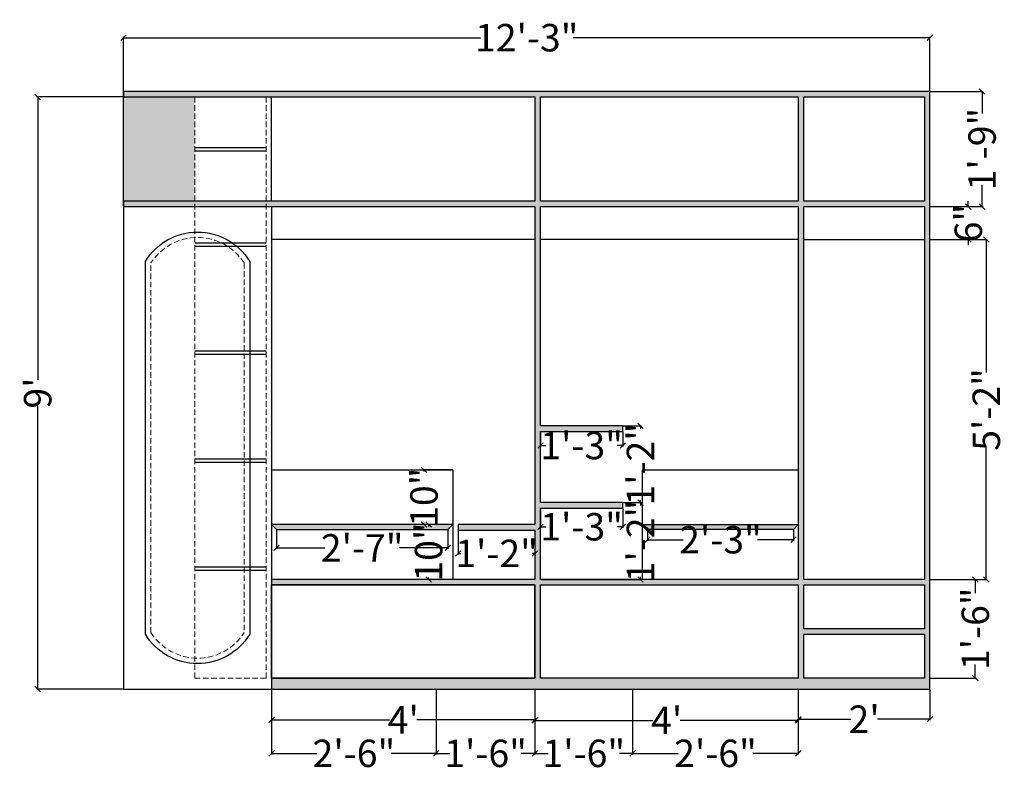
# Model space of a CAD drawing. Units: inches. Extents: x 1441 to 1633, y 516 to 722.
# Tile 1 of 2: x 1441 to 1620, y 516 to 653. Entities that reach past the tile are written whole.
import ezdxf

# ---------------------------------------------------------------- set-up
doc = ezdxf.new("R2010")
doc.units = ezdxf.units.IN
doc.header["$LTSCALE"] = 2
doc.header["$MEASUREMENT"] = 0
doc.linetypes.add('DASHED', pattern=[0.75, 0.5, -0.25])
for name, color, linetype, lineweight in [('A-ANNO-DIMS', 2, 'Continuous', 18), ('A-FURN', 7, 'Continuous', 25), ('A-FURN-OVHD', 4, 'DASHED', 18), ('A-FURN-PATT', 252, 'Continuous', 13)]:
    doc.layers.add(name, color=color, linetype=linetype, lineweight=lineweight)
doc.styles.get("Standard").update_dxf_attribs({"font": 'arial.ttf'})
doc.dimstyles.get("Standard").update_dxf_attribs({"dimtxt": 5, "dimasz": 1, "dimexe": 0.18, "dimexo": 0.0625, "dimgap": 0.09, "dimtad": 0, "dimdec": 0, "dimzin": 0, "dimdsep": 46, "dimlunit": 4, "dimtxsty": 'Standard', "dimblk": 'OBLIQUE', "dimcen": 0.09, "dimadec": 0, "dimazin": 0, "dimtfac": 1, "dimtdec": 0, "dimtofl": 0, "dimtmove": 0, "dimatfit": 3, "dimldrblk": 'OBLIQUE', "dimfxl": 1, "dimtolj": 1, "dimtzin": 0, "dimarcsym": 1})

# ---------------------------------------------------------------- blocks, each defined once
blk = doc.blocks.new('_Oblique')
at = {"color": 0, "linetype": 'ByBlock', "lineweight": -2}
blk.add_line((-0.5, -0.5), (0.5, 0.5), dxfattribs=at)
blk = doc.blocks.new('*D3')
at = {"layer": 'A-ANNO-DIMS', "color": 0, "lineweight": -2, "transparency": 16777216}
for p, q in [((1520.66, 559.91), (1520.66, 555.53)), ((1534.66, 559.91), (1534.66, 555.53)), ((1520.66, 555.71), (1521.16, 555.71)), ((1534.66, 555.71), (1534.16, 555.71))]:
    blk.add_line(p, q, dxfattribs=at)
at = {"layer": 'Defpoints', "color": 0, "transparency": 16777216}
for p in [(1520.66, 559.97), (1534.66, 559.97), (1534.66, 555.71)]:
    blk.add_point(p, dxfattribs=at)
at = {"layer": 'A-ANNO-DIMS', "color": 0, "lineweight": -2, "transparency": 16777216, "rotation": 180}
blk.add_blockref('_Oblique', (1520.66, 555.71), dxfattribs=at)
at = {"layer": 'A-ANNO-DIMS', "color": 0, "lineweight": -2, "transparency": 16777216}
blk.add_blockref('_Oblique', (1534.66, 555.71), dxfattribs=at)
at = {"layer": 'A-ANNO-DIMS', "color": 0, "transparency": 16777216, "insert": (1527.66, 555.71), "char_height": 5, "attachment_point": 5}
blk.add_mtext('\\A1;1\'-2"', dxfattribs=at)
blk = doc.blocks.new('*D4')
at = {"layer": 'A-ANNO-DIMS', "color": 0, "lineweight": -2, "transparency": 16777216}
for p, q in [((1535.66, 563.91), (1535.66, 560.39)), ((1550.66, 563.91), (1550.66, 560.39)), ((1535.66, 560.57), (1536.66, 560.57)), ((1550.66, 560.57), (1549.66, 560.57))]:
    blk.add_line(p, q, dxfattribs=at)
at = {"layer": 'Defpoints', "color": 0, "transparency": 16777216}
for p in [(1535.66, 563.97), (1550.66, 563.97), (1550.66, 560.57)]:
    blk.add_point(p, dxfattribs=at)
at = {"layer": 'A-ANNO-DIMS', "color": 0, "lineweight": -2, "transparency": 16777216, "rotation": 180}
blk.add_blockref('_Oblique', (1535.66, 560.57), dxfattribs=at)
at = {"layer": 'A-ANNO-DIMS', "color": 0, "lineweight": -2, "transparency": 16777216}
blk.add_blockref('_Oblique', (1550.66, 560.57), dxfattribs=at)
at = {"layer": 'A-ANNO-DIMS', "color": 0, "transparency": 16777216, "insert": (1543.16, 560.57), "char_height": 5, "attachment_point": 5}
blk.add_mtext('\\A1;1\'-3"', dxfattribs=at)
blk = doc.blocks.new('*D5')
at = {"layer": 'A-ANNO-DIMS', "color": 0, "lineweight": -2, "transparency": 16777216}
for p, q in [((1535.66, 577.91), (1535.66, 575.21)), ((1550.66, 577.91), (1550.66, 575.21)), ((1535.66, 575.39), (1536.66, 575.39)), ((1550.66, 575.39), (1549.66, 575.39))]:
    blk.add_line(p, q, dxfattribs=at)
at = {"layer": 'Defpoints', "color": 0, "transparency": 16777216}
for p in [(1535.66, 577.97), (1550.66, 577.97), (1550.66, 575.39)]:
    blk.add_point(p, dxfattribs=at)
at = {"layer": 'A-ANNO-DIMS', "color": 0, "lineweight": -2, "transparency": 16777216, "rotation": 180}
blk.add_blockref('_Oblique', (1535.66, 575.39), dxfattribs=at)
at = {"layer": 'A-ANNO-DIMS', "color": 0, "lineweight": -2, "transparency": 16777216}
blk.add_blockref('_Oblique', (1550.66, 575.39), dxfattribs=at)
at = {"layer": 'A-ANNO-DIMS', "color": 0, "transparency": 16777216, "insert": (1543.16, 575.39), "char_height": 5, "attachment_point": 5}
blk.add_mtext('\\A1;1\'-3"', dxfattribs=at)
blk = doc.blocks.new('*D6')
at = {"layer": 'A-ANNO-DIMS', "color": 0, "lineweight": -2, "transparency": 16777216}
for p, q in [((1555.18, 559.99), (1555.18, 558.03)), ((1581.77, 559.99), (1581.77, 558.03)), ((1555.18, 558.21), (1561.69, 558.21)), ((1581.77, 558.21), (1575.25, 558.21))]:
    blk.add_line(p, q, dxfattribs=at)
at = {"layer": 'Defpoints', "color": 0, "transparency": 16777216}
for p in [(1555.18, 560.05), (1581.77, 560.05), (1555.18, 558.21)]:
    blk.add_point(p, dxfattribs=at)
at = {"layer": 'A-ANNO-DIMS', "color": 0, "lineweight": -2, "transparency": 16777216, "rotation": 180}
blk.add_blockref('_Oblique', (1555.18, 558.21), dxfattribs=at)
at = {"layer": 'A-ANNO-DIMS', "color": 0, "lineweight": -2, "transparency": 16777216}
blk.add_blockref('_Oblique', (1581.77, 558.21), dxfattribs=at)
at = {"layer": 'A-ANNO-DIMS', "color": 0, "transparency": 16777216, "insert": (1568.47, 558.21), "char_height": 5, "attachment_point": 5}
blk.add_mtext('\\A1;2\'-3"', dxfattribs=at)
blk = doc.blocks.new('*D7')
at = {"layer": 'A-ANNO-DIMS', "color": 0, "lineweight": -2, "transparency": 16777216}
for p, q in [((1487.55, 559.99), (1487.55, 556.54)), ((1518.77, 559.99), (1518.77, 556.54)), ((1487.55, 556.72), (1496.38, 556.72)), ((1518.77, 556.72), (1509.94, 556.72))]:
    blk.add_line(p, q, dxfattribs=at)
at = {"layer": 'Defpoints', "color": 0, "transparency": 16777216}
for p in [(1487.55, 560.05), (1518.77, 560.05), (1518.77, 556.72)]:
    blk.add_point(p, dxfattribs=at)
at = {"layer": 'A-ANNO-DIMS', "color": 0, "lineweight": -2, "transparency": 16777216, "rotation": 180}
blk.add_blockref('_Oblique', (1487.55, 556.72), dxfattribs=at)
at = {"layer": 'A-ANNO-DIMS', "color": 0, "lineweight": -2, "transparency": 16777216}
blk.add_blockref('_Oblique', (1518.77, 556.72), dxfattribs=at)
at = {"layer": 'A-ANNO-DIMS', "color": 0, "transparency": 16777216, "insert": (1503.16, 556.72), "char_height": 5, "attachment_point": 5}
blk.add_mtext('\\A1;2\'-7"', dxfattribs=at)
blk = doc.blocks.new('*D8')
at = {"layer": 'A-ANNO-DIMS', "color": 0, "lineweight": -2, "transparency": 16777216}
for p, q in [((1534.66, 530.91), (1534.66, 525.07)), ((1582.66, 530.91), (1582.66, 525.07)), ((1534.66, 525.25), (1556.17, 525.25)), ((1582.66, 525.25), (1561.15, 525.25))]:
    blk.add_line(p, q, dxfattribs=at)
at = {"layer": 'Defpoints', "color": 0, "transparency": 16777216}
for p in [(1534.66, 530.97), (1582.66, 530.97), (1582.66, 525.25)]:
    blk.add_point(p, dxfattribs=at)
at = {"layer": 'A-ANNO-DIMS', "color": 0, "lineweight": -2, "transparency": 16777216, "rotation": 180}
blk.add_blockref('_Oblique', (1534.66, 525.25), dxfattribs=at)
at = {"layer": 'A-ANNO-DIMS', "color": 0, "lineweight": -2, "transparency": 16777216}
blk.add_blockref('_Oblique', (1582.66, 525.25), dxfattribs=at)
at = {"layer": 'A-ANNO-DIMS', "color": 0, "transparency": 16777216, "insert": (1558.66, 525.25), "char_height": 5, "attachment_point": 5}
blk.add_mtext("\\A1;4'", dxfattribs=at)
blk = doc.blocks.new('*D9')
at = {"layer": 'A-ANNO-DIMS', "color": 0, "lineweight": -2, "transparency": 16777216}
for p, q in [((1582.66, 530.91), (1582.66, 525.29)), ((1606.66, 530.91), (1606.66, 525.29)), ((1582.66, 525.47), (1592.23, 525.47)), ((1606.66, 525.47), (1597.1, 525.47))]:
    blk.add_line(p, q, dxfattribs=at)
at = {"layer": 'Defpoints', "color": 0, "transparency": 16777216}
for p in [(1582.66, 530.97), (1606.66, 530.97), (1606.66, 525.47)]:
    blk.add_point(p, dxfattribs=at)
at = {"layer": 'A-ANNO-DIMS', "color": 0, "lineweight": -2, "transparency": 16777216, "rotation": 180}
blk.add_blockref('_Oblique', (1582.66, 525.47), dxfattribs=at)
at = {"layer": 'A-ANNO-DIMS', "color": 0, "lineweight": -2, "transparency": 16777216}
blk.add_blockref('_Oblique', (1606.66, 525.47), dxfattribs=at)
at = {"layer": 'A-ANNO-DIMS', "color": 0, "transparency": 16777216, "insert": (1594.66, 525.47), "char_height": 5, "attachment_point": 5}
blk.add_mtext("\\A1;2'", dxfattribs=at)
blk = doc.blocks.new('*D10')
at = {"layer": 'A-ANNO-DIMS', "color": 0, "lineweight": -2, "transparency": 16777216}
for p, q in [((1486.66, 530.91), (1486.66, 525.17)), ((1534.66, 530.91), (1534.66, 525.17)), ((1486.66, 525.35), (1508.17, 525.35)), ((1534.66, 525.35), (1513.15, 525.35))]:
    blk.add_line(p, q, dxfattribs=at)
at = {"layer": 'Defpoints', "color": 0, "transparency": 16777216}
for p in [(1486.66, 530.97), (1534.66, 530.97), (1534.66, 525.35)]:
    blk.add_point(p, dxfattribs=at)
at = {"layer": 'A-ANNO-DIMS', "color": 0, "lineweight": -2, "transparency": 16777216, "rotation": 180}
blk.add_blockref('_Oblique', (1486.66, 525.35), dxfattribs=at)
at = {"layer": 'A-ANNO-DIMS', "color": 0, "lineweight": -2, "transparency": 16777216}
blk.add_blockref('_Oblique', (1534.66, 525.35), dxfattribs=at)
at = {"layer": 'A-ANNO-DIMS', "color": 0, "transparency": 16777216, "insert": (1510.66, 525.35), "char_height": 5, "attachment_point": 5}
blk.add_mtext("\\A1;4'", dxfattribs=at)
blk = doc.blocks.new('*D11')
at = {"layer": 'A-ANNO-DIMS', "color": 0, "lineweight": -2, "transparency": 16777216}
for p, q in [((1606.73, 550.97), (1615.1, 550.97)), ((1614.92, 550.97), (1614.92, 548.47)), ((1614.92, 532.97), (1614.92, 535.47)), ((1606.73, 532.97), (1615.1, 532.97))]:
    blk.add_line(p, q, dxfattribs=at)
at = {"layer": 'Defpoints', "color": 0, "transparency": 16777216}
for p in [(1606.66, 550.97), (1614.92, 550.97), (1606.66, 532.97)]:
    blk.add_point(p, dxfattribs=at)
at = {"layer": 'A-ANNO-DIMS', "color": 0, "lineweight": -2, "transparency": 16777216}
for p, rotation in [((1614.92, 550.97), 90), ((1614.92, 532.97), 270)]:
    blk.add_blockref('_Oblique', p, dxfattribs=dict(at, rotation=rotation))
at = {"layer": 'A-ANNO-DIMS', "color": 0, "transparency": 16777216, "insert": (1614.92, 541.97), "char_height": 5, "attachment_point": 5, "rotation": 90}
blk.add_mtext('\\A1;1\'-6"', dxfattribs=at)
blk = doc.blocks.new('*D12')
at = {"layer": 'A-ANNO-DIMS', "color": 0, "lineweight": -2, "transparency": 16777216}
for p, q in [((1606.73, 612.97), (1617.11, 612.97)), ((1616.93, 612.97), (1616.93, 588.71)), ((1616.93, 550.97), (1616.93, 575.24)), ((1606.73, 550.97), (1617.11, 550.97))]:
    blk.add_line(p, q, dxfattribs=at)
at = {"layer": 'Defpoints', "color": 0, "transparency": 16777216}
for p in [(1606.66, 612.97), (1616.93, 612.97), (1606.66, 550.97)]:
    blk.add_point(p, dxfattribs=at)
at = {"layer": 'A-ANNO-DIMS', "color": 0, "lineweight": -2, "transparency": 16777216}
for p, rotation in [((1616.93, 612.97), 90), ((1616.93, 550.97), 270)]:
    blk.add_blockref('_Oblique', p, dxfattribs=dict(at, rotation=rotation))
at = {"layer": 'A-ANNO-DIMS', "color": 0, "transparency": 16777216, "insert": (1616.93, 581.97), "char_height": 5, "attachment_point": 5, "rotation": 90}
blk.add_mtext('\\A1;5\'-2"', dxfattribs=at)
blk = doc.blocks.new('*D13')
at = {"layer": 'A-ANNO-DIMS', "color": 0, "lineweight": -2, "transparency": 16777216}
for p, q in [((1613.64, 618.97), (1613.64, 619.97)), ((1606.73, 618.97), (1613.82, 618.97)), ((1606.73, 612.97), (1613.82, 612.97)), ((1613.64, 612.97), (1613.64, 611.97))]:
    blk.add_line(p, q, dxfattribs=at)
at = {"layer": 'Defpoints', "color": 0, "transparency": 16777216}
for p in [(1606.66, 618.97), (1613.64, 618.97), (1606.66, 612.97)]:
    blk.add_point(p, dxfattribs=at)
at = {"layer": 'A-ANNO-DIMS', "color": 0, "lineweight": -2, "transparency": 16777216}
for p, rotation in [((1613.64, 618.97), 270), ((1613.64, 612.97), 90)]:
    blk.add_blockref('_Oblique', p, dxfattribs=dict(at, rotation=rotation))
at = {"layer": 'A-ANNO-DIMS', "color": 0, "transparency": 16777216, "insert": (1613.64, 615.97), "char_height": 5, "attachment_point": 5, "rotation": 90}
blk.add_mtext('\\A1;6"', dxfattribs=at)
blk = doc.blocks.new('*D14')
at = {"layer": 'A-ANNO-DIMS', "color": 0, "lineweight": -2, "transparency": 16777216}
for p, q in [((1606.73, 639.97), (1616.33, 639.97)), ((1616.15, 639.97), (1616.15, 635.97)), ((1616.15, 618.97), (1616.15, 622.97)), ((1606.73, 618.97), (1616.33, 618.97))]:
    blk.add_line(p, q, dxfattribs=at)
at = {"layer": 'Defpoints', "color": 0, "transparency": 16777216}
for p in [(1606.66, 639.97), (1616.15, 639.97), (1606.66, 618.97)]:
    blk.add_point(p, dxfattribs=at)
at = {"layer": 'A-ANNO-DIMS', "color": 0, "lineweight": -2, "transparency": 16777216}
for p, rotation in [((1616.15, 639.97), 90), ((1616.15, 618.97), 270)]:
    blk.add_blockref('_Oblique', p, dxfattribs=dict(at, rotation=rotation))
at = {"layer": 'A-ANNO-DIMS', "color": 0, "transparency": 16777216, "insert": (1616.15, 629.47), "char_height": 5, "attachment_point": 5, "rotation": 90}
blk.add_mtext('\\A1;1\'-9"', dxfattribs=at)
blk = doc.blocks.new('*D15')
at = {"layer": 'A-ANNO-DIMS', "color": 0, "lineweight": -2, "transparency": 16777216}
for p, q in [((1459.66, 640.04), (1459.66, 649.97)), ((1459.66, 649.79), (1524.72, 649.79)), ((1606.66, 649.79), (1541.61, 649.79)), ((1606.66, 640.04), (1606.66, 649.97))]:
    blk.add_line(p, q, dxfattribs=at)
at = {"layer": 'Defpoints', "color": 0, "transparency": 16777216}
for p in [(1459.66, 649.79), (1459.66, 639.97), (1606.66, 639.97)]:
    blk.add_point(p, dxfattribs=at)
at = {"layer": 'A-ANNO-DIMS', "color": 0, "lineweight": -2, "transparency": 16777216, "rotation": 180}
blk.add_blockref('_Oblique', (1459.66, 649.79), dxfattribs=at)
at = {"layer": 'A-ANNO-DIMS', "color": 0, "lineweight": -2, "transparency": 16777216}
blk.add_blockref('_Oblique', (1606.66, 649.79), dxfattribs=at)
at = {"layer": 'A-ANNO-DIMS', "color": 0, "transparency": 16777216, "insert": (1533.16, 649.79), "char_height": 5, "attachment_point": 5}
blk.add_mtext('\\A1;12\'-3"', dxfattribs=at)
blk = doc.blocks.new('*D16')
at = {"layer": 'A-ANNO-DIMS', "color": 0, "lineweight": -2, "transparency": 16777216}
for p, q in [((1459.6, 638.97), (1443.84, 638.97)), ((1444.02, 638.97), (1444.02, 587.37)), ((1444.02, 530.97), (1444.02, 582.58)), ((1459.6, 530.97), (1443.84, 530.97))]:
    blk.add_line(p, q, dxfattribs=at)
at = {"layer": 'Defpoints', "color": 0, "transparency": 16777216}
for p in [(1459.66, 638.97), (1444.02, 530.97), (1459.66, 530.97)]:
    blk.add_point(p, dxfattribs=at)
at = {"layer": 'A-ANNO-DIMS', "color": 0, "lineweight": -2, "transparency": 16777216}
for p, rotation in [((1444.02, 638.97), 90), ((1444.02, 530.97), 270)]:
    blk.add_blockref('_Oblique', p, dxfattribs=dict(at, rotation=rotation))
at = {"layer": 'A-ANNO-DIMS', "color": 0, "transparency": 16777216, "insert": (1444.02, 584.97), "char_height": 5, "attachment_point": 5, "rotation": 90}
blk.add_mtext("\\A1;9'", dxfattribs=at)
blk = doc.blocks.new('*D17')
at = {"layer": 'A-ANNO-DIMS', "color": 0, "lineweight": -2, "transparency": 16777216}
for p, q in [((1486.66, 530.91), (1486.66, 519.06)), ((1516.66, 530.91), (1516.66, 519.06)), ((1486.66, 519.24), (1494.88, 519.24)), ((1516.66, 519.24), (1508.44, 519.24))]:
    blk.add_line(p, q, dxfattribs=at)
at = {"layer": 'Defpoints', "color": 0, "transparency": 16777216}
for p in [(1486.66, 530.97), (1516.66, 530.97), (1516.66, 519.24)]:
    blk.add_point(p, dxfattribs=at)
at = {"layer": 'A-ANNO-DIMS', "color": 0, "lineweight": -2, "transparency": 16777216, "rotation": 180}
blk.add_blockref('_Oblique', (1486.66, 519.24), dxfattribs=at)
at = {"layer": 'A-ANNO-DIMS', "color": 0, "lineweight": -2, "transparency": 16777216}
blk.add_blockref('_Oblique', (1516.66, 519.24), dxfattribs=at)
at = {"layer": 'A-ANNO-DIMS', "color": 0, "transparency": 16777216, "insert": (1501.66, 519.24), "char_height": 5, "attachment_point": 5}
blk.add_mtext('\\A1;2\'-6"', dxfattribs=at)
blk = doc.blocks.new('*D18')
at = {"layer": 'A-ANNO-DIMS', "color": 0, "lineweight": -2, "transparency": 16777216}
for p, q in [((1552.46, 530.91), (1552.46, 519.06)), ((1582.66, 530.91), (1582.66, 519.06)), ((1552.46, 519.24), (1560.78, 519.24)), ((1582.66, 519.24), (1574.34, 519.24))]:
    blk.add_line(p, q, dxfattribs=at)
at = {"layer": 'Defpoints', "color": 0, "transparency": 16777216}
for p in [(1552.46, 530.97), (1582.66, 530.97), (1552.46, 519.24)]:
    blk.add_point(p, dxfattribs=at)
at = {"layer": 'A-ANNO-DIMS', "color": 0, "lineweight": -2, "transparency": 16777216, "rotation": 180}
blk.add_blockref('_Oblique', (1552.46, 519.24), dxfattribs=at)
at = {"layer": 'A-ANNO-DIMS', "color": 0, "lineweight": -2, "transparency": 16777216}
blk.add_blockref('_Oblique', (1582.66, 519.24), dxfattribs=at)
at = {"layer": 'A-ANNO-DIMS', "color": 0, "transparency": 16777216, "insert": (1567.56, 519.24), "char_height": 5, "attachment_point": 5}
blk.add_mtext('\\A1;2\'-6"', dxfattribs=at)
blk = doc.blocks.new('*D19')
at = {"layer": 'A-ANNO-DIMS', "color": 0, "lineweight": -2, "transparency": 16777216}
for p, q in [((1534.66, 530.91), (1534.66, 519.06)), ((1534.66, 519.24), (1537.06, 519.24)), ((1552.46, 519.24), (1550.06, 519.24)), ((1552.46, 519.31), (1552.46, 519.42))]:
    blk.add_line(p, q, dxfattribs=at)
at = {"layer": 'Defpoints', "color": 0, "transparency": 16777216}
for p in [(1534.66, 530.97), (1552.46, 519.24), (1552.46, 519.24)]:
    blk.add_point(p, dxfattribs=at)
at = {"layer": 'A-ANNO-DIMS', "color": 0, "lineweight": -2, "transparency": 16777216, "rotation": 180}
blk.add_blockref('_Oblique', (1534.66, 519.24), dxfattribs=at)
at = {"layer": 'A-ANNO-DIMS', "color": 0, "lineweight": -2, "transparency": 16777216}
blk.add_blockref('_Oblique', (1552.46, 519.24), dxfattribs=at)
at = {"layer": 'A-ANNO-DIMS', "color": 0, "transparency": 16777216, "insert": (1543.56, 519.24), "char_height": 5, "attachment_point": 5}
blk.add_mtext('\\A1;1\'-6"', dxfattribs=at)
blk = doc.blocks.new('*D20')
at = {"layer": 'A-ANNO-DIMS', "color": 0, "lineweight": -2, "transparency": 16777216}
for p, q in [((1534.66, 530.91), (1534.66, 519.06)), ((1516.66, 519.31), (1516.66, 519.42)), ((1516.66, 519.24), (1519.16, 519.24)), ((1534.66, 519.24), (1532.16, 519.24))]:
    blk.add_line(p, q, dxfattribs=at)
at = {"layer": 'Defpoints', "color": 0, "transparency": 16777216}
for p in [(1534.66, 530.97), (1516.66, 519.24), (1516.66, 519.24)]:
    blk.add_point(p, dxfattribs=at)
at = {"layer": 'A-ANNO-DIMS', "color": 0, "lineweight": -2, "transparency": 16777216, "rotation": 180}
blk.add_blockref('_Oblique', (1516.66, 519.24), dxfattribs=at)
at = {"layer": 'A-ANNO-DIMS', "color": 0, "lineweight": -2, "transparency": 16777216}
blk.add_blockref('_Oblique', (1534.66, 519.24), dxfattribs=at)
at = {"layer": 'A-ANNO-DIMS', "color": 0, "transparency": 16777216, "insert": (1525.66, 519.24), "char_height": 5, "attachment_point": 5}
blk.add_mtext('\\A1;1\'-6"', dxfattribs=at)
blk = doc.blocks.new('*D21')
at = {"layer": 'A-ANNO-DIMS', "color": 0, "lineweight": -2, "transparency": 16777216}
for p, q in [((1519.6, 560.97), (1515.09, 560.97)), ((1515.27, 560.97), (1515.27, 560.65)), ((1519.6, 550.97), (1515.09, 550.97)), ((1515.27, 550.97), (1515.27, 551.3))]:
    blk.add_line(p, q, dxfattribs=at)
at = {"layer": 'Defpoints', "color": 0, "transparency": 16777216}
for p in [(1519.66, 560.97), (1515.27, 550.97), (1519.66, 550.97)]:
    blk.add_point(p, dxfattribs=at)
at = {"layer": 'A-ANNO-DIMS', "color": 0, "lineweight": -2, "transparency": 16777216}
for p, rotation in [((1515.27, 560.97), 90), ((1515.27, 550.97), 270)]:
    blk.add_blockref('_Oblique', p, dxfattribs=dict(at, rotation=rotation))
at = {"layer": 'A-ANNO-DIMS', "color": 0, "transparency": 16777216, "insert": (1515.27, 555.97), "char_height": 5, "attachment_point": 5, "rotation": 90}
blk.add_mtext('\\A1;10"', dxfattribs=at)
blk = doc.blocks.new('*D22')
at = {"layer": 'A-ANNO-DIMS', "color": 0, "lineweight": -2, "transparency": 16777216}
for p, q in [((1519.6, 570.97), (1514.25, 570.97)), ((1514.43, 570.97), (1514.43, 570.65)), ((1519.6, 560.97), (1514.25, 560.97)), ((1514.43, 560.97), (1514.43, 561.3))]:
    blk.add_line(p, q, dxfattribs=at)
at = {"layer": 'Defpoints', "color": 0, "transparency": 16777216}
for p in [(1519.66, 570.97), (1514.43, 560.97), (1519.66, 560.97)]:
    blk.add_point(p, dxfattribs=at)
at = {"layer": 'A-ANNO-DIMS', "color": 0, "lineweight": -2, "transparency": 16777216}
for p, rotation in [((1514.43, 570.97), 90), ((1514.43, 560.97), 270)]:
    blk.add_blockref('_Oblique', p, dxfattribs=dict(at, rotation=rotation))
at = {"layer": 'A-ANNO-DIMS', "color": 0, "transparency": 16777216, "insert": (1514.43, 565.97), "char_height": 5, "attachment_point": 5, "rotation": 90}
blk.add_mtext('\\A1;10"', dxfattribs=at)
blk = doc.blocks.new('*D23')
at = {"layer": 'A-ANNO-DIMS', "color": 0, "lineweight": -2, "transparency": 16777216}
for p, q in [((1550.73, 578.97), (1554.07, 578.97)), ((1553.89, 578.97), (1553.89, 578.47)), ((1553.89, 564.97), (1553.89, 565.47)), ((1550.73, 564.97), (1554.07, 564.97))]:
    blk.add_line(p, q, dxfattribs=at)
at = {"layer": 'Defpoints', "color": 0, "transparency": 16777216}
for p in [(1550.66, 578.97), (1553.89, 578.97), (1550.66, 564.97)]:
    blk.add_point(p, dxfattribs=at)
at = {"layer": 'A-ANNO-DIMS', "color": 0, "lineweight": -2, "transparency": 16777216}
for p, rotation in [((1553.89, 578.97), 90), ((1553.89, 564.97), 270)]:
    blk.add_blockref('_Oblique', p, dxfattribs=dict(at, rotation=rotation))
at = {"layer": 'A-ANNO-DIMS', "color": 0, "transparency": 16777216, "insert": (1553.89, 571.97), "char_height": 5, "attachment_point": 5, "rotation": 90}
blk.add_mtext('\\A1;1\'-2"', dxfattribs=at)
blk = doc.blocks.new('*D24')
at = {"layer": 'A-ANNO-DIMS', "color": 0, "lineweight": -2, "transparency": 16777216}
for p, q in [((1550.73, 564.97), (1554.07, 564.97)), ((1553.89, 564.97), (1553.89, 564.47)), ((1535.73, 550.97), (1554.07, 550.97)), ((1553.89, 550.97), (1553.89, 551.47))]:
    blk.add_line(p, q, dxfattribs=at)
at = {"layer": 'Defpoints', "color": 0, "transparency": 16777216}
for p in [(1550.66, 564.97), (1535.66, 550.97), (1553.89, 550.97)]:
    blk.add_point(p, dxfattribs=at)
at = {"layer": 'A-ANNO-DIMS', "color": 0, "lineweight": -2, "transparency": 16777216}
for p, rotation in [((1553.89, 564.97), 90), ((1553.89, 550.97), 270)]:
    blk.add_blockref('_Oblique', p, dxfattribs=dict(at, rotation=rotation))
at = {"layer": 'A-ANNO-DIMS', "color": 0, "transparency": 16777216, "insert": (1553.89, 557.97), "char_height": 5, "attachment_point": 5, "rotation": 90}
blk.add_mtext('\\A1;1\'-2"', dxfattribs=at)

msp = doc.modelspace()

# ---------------------------------------------------------------- hatches: boundary and pattern name
at = {"layer": 'A-FURN-PATT'}
h = msp.add_hatch(color=256, dxfattribs=at)
h.dxf.hatch_style = 1
h.paths.add_polyline_path([(1606.66, 550.97), (1606.66, 612.97), (1606.66, 618.97), (1606.66, 639.97), (1459.66, 639.97), (1459.66, 638.97), (1534.66, 638.97), (1534.66, 619.97), (1459.66, 619.97), (1459.66, 618.97), (1534.66, 618.97), (1534.66, 560.97), (1520.66, 560.97), (1520.66, 559.97), (1534.66, 559.97), (1534.66, 550.97), (1486.66, 550.97), (1486.66, 549.97), (1534.66, 549.97), (1534.66, 532.97), (1486.66, 532.97), (1486.66, 530.97), (1534.66, 530.97), (1582.66, 530.97), (1606.66, 530.97), (1606.66, 532.97)])
h.paths.add_polyline_path([(1535.66, 549.97), (1582.66, 549.97), (1582.66, 532.97), (1535.66, 532.97)], flags=16)
h.paths.add_polyline_path([(1535.66, 550.97), (1535.66, 563.97), (1550.66, 563.97), (1550.66, 564.97), (1535.66, 564.97), (1535.66, 577.97), (1550.66, 577.97), (1550.66, 578.97), (1535.66, 578.97), (1535.66, 618.97), (1582.66, 618.97), (1582.66, 550.97)], flags=16)
h.paths.add_polyline_path([(1554.28, 560.97), (1582.66, 560.97), (1581.77, 560.05), (1555.18, 560.05)], flags=0)
h.paths.add_polyline_path([(1583.66, 549.97), (1605.66, 549.97), (1605.66, 541.97), (1583.66, 541.97)], flags=16)
h.paths.add_polyline_path([(1583.66, 550.97), (1583.66, 618.97), (1605.66, 618.97), (1605.66, 612.97), (1605.66, 550.97)], flags=16)
h.paths.add_polyline_path([(1583.66, 540.97), (1605.66, 540.97), (1605.66, 532.97), (1583.66, 532.97)], flags=16)
h.paths.add_polyline_path([(1535.66, 619.97), (1535.66, 638.97), (1582.66, 638.97), (1582.66, 619.97)], flags=16)
h.paths.add_polyline_path([(1583.66, 619.97), (1583.66, 638.97), (1605.66, 638.97), (1605.66, 619.97)], flags=16)
h.paths.add_polyline_path([(1582.66, 618.97), (1535.66, 618.97), (1535.66, 578.97), (1550.66, 578.97), (1550.66, 577.97), (1535.66, 577.97), (1535.66, 564.97), (1550.66, 564.97), (1550.66, 563.97), (1535.66, 563.97), (1535.66, 550.97), (1582.66, 550.97)], flags=0)
h = msp.add_hatch(color=256, dxfattribs=at)
h.dxf.hatch_style = 1
h.paths.add_polyline_path([(1472.66, 638.97), (1459.66, 638.97), (1459.66, 619.97), (1472.66, 619.97)])
h = msp.add_hatch(color=256, dxfattribs=at)
h.dxf.hatch_style = 1
h.paths.add_polyline_path([(1582.66, 560.97), (1554.28, 560.97), (1555.18, 560.05), (1581.77, 560.05)])
h.paths.add_polyline_path([(1519.66, 560.97), (1486.66, 560.97), (1487.55, 560.05), (1518.77, 560.05)])

# ---------------------------------------------------------------- linework, layer by layer
at = {"layer": 'A-FURN'}
for p, q in [((1459.66, 618.97), (1459.66, 639.97)), ((1486.66, 619.97), (1486.66, 638.97)), ((1472.66, 629.77), (1485.66, 629.77)), ((1472.66, 629.17), (1485.66, 629.17)), ((1485.66, 619.97), (1472.66, 619.97)), ((1459.66, 618.97), (1459.66, 530.97)), ((1472.66, 612.37), (1485.66, 612.37)), ((1534.66, 612.97), (1486.66, 612.97)), ((1582.66, 612.97), (1535.66, 612.97)), ((1472.66, 611.77), (1485.66, 611.77)), ((1472.66, 592.67), (1485.66, 592.67)), ((1472.66, 592.07), (1485.66, 592.07)), ((1472.66, 572.97), (1485.66, 572.97)), ((1472.66, 572.37), (1485.66, 572.37)), ((1486.66, 560.97), (1487.55, 560.05)), ((1472.66, 553.27), (1485.66, 553.27)), ((1472.66, 552.67), (1485.66, 552.67)), ((1459.66, 530.97), (1486.66, 530.97))]:
    msp.add_line(p, q, dxfattribs=at)
for points in [[(1486.66, 618.97), (1486.66, 530.97), (1534.66, 530.97), (1582.66, 530.97), (1606.66, 530.97), (1606.66, 532.97), (1606.66, 550.97), (1606.66, 612.97), (1606.66, 618.97), (1606.66, 639.97), (1459.66, 639.97), (1459.66, 638.97), (1534.66, 638.97), (1534.66, 619.97), (1459.66, 619.97), (1459.66, 618.97), (1534.66, 618.97), (1534.66, 560.97), (1520.66, 560.97), (1520.66, 559.97), (1534.66, 559.97), (1534.66, 550.97), (1486.66, 550.97)], [(1583.66, 612.97), (1605.66, 612.97), (1605.66, 550.97), (1583.66, 550.97), (1583.66, 618.97), (1605.66, 618.97), (1605.66, 612.97)], [(1486.66, 570.97), (1519.66, 570.97), (1519.66, 550.97)], [(1554.28, 550.97), (1554.28, 570.97), (1582.66, 570.97)], [(1487.55, 560.05), (1518.77, 560.05), (1519.66, 560.97), (1486.66, 560.97)], [(1486.66, 532.97), (1534.66, 532.97), (1534.66, 549.97), (1486.66, 549.97)]]:
    msp.add_lwpolyline(points, dxfattribs=at)
for points in [[(1535.66, 619.97), (1535.66, 638.97), (1582.66, 638.97), (1582.66, 619.97)], [(1583.66, 619.97), (1583.66, 638.97), (1605.66, 638.97), (1605.66, 619.97)], [(1535.66, 563.97), (1550.66, 563.97), (1550.66, 564.97), (1535.66, 564.97), (1535.66, 577.97), (1550.66, 577.97), (1550.66, 578.97), (1535.66, 578.97), (1535.66, 618.97), (1582.66, 618.97), (1582.66, 550.97), (1535.66, 550.97)], [(1582.66, 560.97), (1581.77, 560.05), (1555.18, 560.05), (1554.28, 560.97)], [(1486.66, 549.97), (1534.66, 549.97), (1534.66, 532.97), (1486.66, 532.97)], [(1535.66, 532.97), (1535.66, 549.97), (1582.66, 549.97), (1582.66, 532.97)], [(1605.66, 541.97), (1583.66, 541.97), (1583.66, 549.97), (1605.66, 549.97)], [(1605.66, 532.97), (1583.66, 532.97), (1583.66, 540.97), (1605.66, 540.97)]]:
    msp.add_lwpolyline(points, close=True, dxfattribs=at)
msp.add_lwpolyline([(1482.66, 608.97), (1482.66, 540.97, -0.564803), (1463.66, 540.97), (1463.66, 608.97, -0.564803)], format="xyb", close=True, dxfattribs=at)
at = {"layer": 'A-FURN-OVHD'}
msp.add_lwpolyline([(1472.66, 638.97), (1485.66, 638.97), (1485.66, 532.97), (1472.66, 532.97)], close=True, dxfattribs=at)
msp.add_lwpolyline([(1481.66, 608.69), (1481.66, 541.26, -0.547158), (1464.66, 541.26), (1464.66, 608.69, -0.547158)], format="xyb", close=True, dxfattribs=at)

# ---------------------------------------------------------------- dimensions: what is measured, and where the dimension line sits
at = {"layer": 'A-ANNO-DIMS'}
for base, p1, p2, picture, middle in [((1459.66, 649.79), (1606.66, 639.97), (1459.66, 639.97), '*D15', (1533.16, 649.79)), ((1550.66, 575.39), (1535.66, 577.97), (1550.66, 577.97), '*D5', (1543.16, 575.39)), ((1550.66, 560.57), (1535.66, 563.97), (1550.66, 563.97), '*D4', (1543.16, 560.57)), ((1518.77, 556.72), (1487.55, 560.05), (1518.77, 560.05), '*D7', (1503.16, 556.72)), ((1534.66, 555.71), (1520.66, 559.97), (1534.66, 559.97), '*D3', (1527.66, 555.71)), ((1555.18, 558.21), (1581.77, 560.05), (1555.18, 560.05), '*D6', (1568.47, 558.21)), ((1534.66, 525.35), (1486.66, 530.97), (1534.66, 530.97), '*D10', (1510.66, 525.35)), ((1516.66, 519.24), (1486.66, 530.97), (1516.66, 530.97), '*D17', (1501.66, 519.24)), ((1516.66, 519.24), (1534.66, 530.97), (1516.66, 519.24), '*D20', (1525.66, 519.24)), ((1582.66, 525.25), (1534.66, 530.97), (1582.66, 530.97), '*D8', (1558.66, 525.25)), ((1552.46, 519.24), (1534.66, 530.97), (1552.46, 519.24), '*D19', (1543.56, 519.24)), ((1552.46, 519.24), (1582.66, 530.97), (1552.46, 530.97), '*D18', (1567.56, 519.24)), ((1606.66, 525.47), (1582.66, 530.97), (1606.66, 530.97), '*D9', (1594.66, 525.47))]:
    dim = msp.add_linear_dim(base=base, p1=p1, p2=p2, dimstyle='Standard', override={"dimclrd": 0, "dimclre": 0, "dimclrt": 0}, dxfattribs=at)
    dim.commit()
    dim.dimension.update_dxf_attribs({"geometry": picture, "text_midpoint": middle})
for base, p1, p2, picture, middle in [((1444.02, 530.97), (1459.66, 638.97), (1459.66, 530.97), '*D16', (1444.02, 584.97)), ((1616.15, 639.97), (1606.66, 618.97), (1606.66, 639.97), '*D14', (1616.15, 629.47)), ((1613.64, 618.97), (1606.66, 612.97), (1606.66, 618.97), '*D13', (1613.64, 615.97)), ((1616.93, 612.97), (1606.66, 550.97), (1606.66, 612.97), '*D12', (1616.93, 581.97)), ((1553.89, 578.97), (1550.66, 564.97), (1550.66, 578.97), '*D23', (1553.89, 571.97)), ((1514.43, 560.97), (1519.66, 570.97), (1519.66, 560.97), '*D22', (1514.43, 565.97)), ((1553.89, 550.97), (1550.66, 564.97), (1535.66, 550.97), '*D24', (1553.89, 557.97)), ((1515.27, 550.97), (1519.66, 560.97), (1519.66, 550.97), '*D21', (1515.27, 555.97)), ((1614.92, 550.97), (1606.66, 532.97), (1606.66, 550.97), '*D11', (1614.92, 541.97))]:
    dim = msp.add_linear_dim(base=base, p1=p1, p2=p2, angle=90, dimstyle='Standard', override={"dimclrd": 0, "dimclre": 0, "dimclrt": 0}, dxfattribs=at)
    dim.commit()
    dim.dimension.update_dxf_attribs({"geometry": picture, "text_midpoint": middle})

doc.saveas('drawing.dxf')
